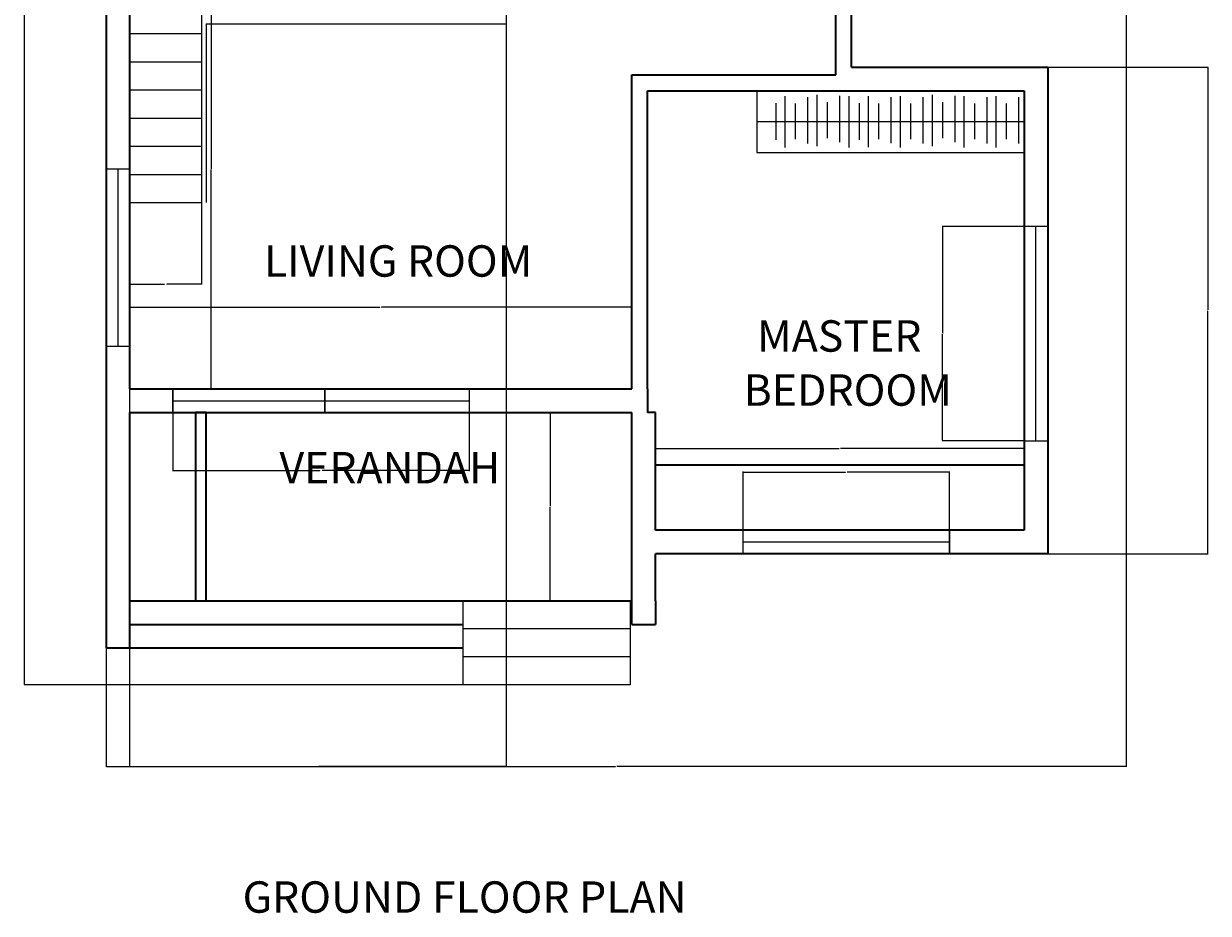
# Model space of a CAD drawing. Units: inches. Extents: x 1741 to 3812, y 9290 to 10023.
# Tile 1 of 5: x 1741 to 2194, y 9290 to 9630. Entities that reach past the tile are written whole.
import ezdxf

# ---------------------------------------------------------------- set-up
doc = ezdxf.new("R2010")
doc.units = ezdxf.units.IN
doc.header["$MEASUREMENT"] = 0
for name, color, linetype, lineweight in [('A-ANNO-DIMS', 2, 'Continuous', 18), ('A-ANNO-TEXT', 7, 'Continuous', 25), ('A-AREA-IDEN', 7, 'Continuous', 18), ('A-FLOR-CASE', 9, 'Continuous', 18), ('A-FLOR-STRS', 3, 'Continuous', 18), ('A-GLAZ', 4, 'Continuous', 18), ('A-WALL', 7, 'Continuous', 35)]:
    doc.layers.add(name, color=color, linetype=linetype, lineweight=lineweight)
doc.styles.get("Standard").update_dxf_attribs({"font": 'arial.ttf'})
doc.dimstyles.get("Standard").update_dxf_attribs({"dimtxt": 0.18, "dimasz": 0.18, "dimexe": 0.18, "dimexo": 0.0625, "dimgap": 0.09, "dimtad": 0, "dimtih": 1, "dimtoh": 1, "dimdec": 4, "dimzin": 0, "dimdsep": 46, "dimtxsty": 'Standard', "dimcen": 0.09, "dimadec": 0, "dimazin": 0, "dimtfac": 1, "dimtdec": 4, "dimtofl": 0, "dimtmove": 0, "dimatfit": 3, "dimfxl": 1, "dimtolj": 1, "dimtzin": 0, "dimarcsym": 0})

# ---------------------------------------------------------------- blocks, each defined once
blk = doc.blocks.new('*D31')
at = {"layer": 'A-ANNO-DIMS', "color": 0, "lineweight": -2, "transparency": 16777216}
for p, q in [((2162.92, 9640.39), (2162.92, 9345.97)), ((1772.92, 9391.39), (1772.92, 9345.97)), ((1773.1, 9346.15), (1967.64, 9346.15)), ((2162.74, 9346.15), (1968.21, 9346.15))]:
    blk.add_line(p, q, dxfattribs=at)
at = {"layer": 'A-ANNO-DIMS', "color": 0, "transparency": 16777216}
for points in [[(1773.1, 9346.18), (1773.1, 9346.12), (1772.92, 9346.15)], [(2162.74, 9346.18), (2162.74, 9346.12), (2162.92, 9346.15)]]:
    blk.add_solid(points, dxfattribs=at)
at = {"layer": 'Defpoints', "color": 0, "transparency": 16777216}
for p in [(2162.92, 9640.45), (1772.92, 9391.45), (2162.92, 9346.15)]:
    blk.add_point(p, dxfattribs=at)
at = {"layer": 'A-ANNO-DIMS', "color": 0, "transparency": 16777216, "insert": (1967.92, 9346.15), "char_height": 0.18, "attachment_point": 5}
blk.add_mtext('\\A1;390', dxfattribs=at)
blk = doc.blocks.new('*D32')
at = {"layer": 'A-ANNO-DIMS', "color": 0, "lineweight": -2, "transparency": 16777216}
for p, q in [((1844.86, 9901.45), (1741.54, 9901.45)), ((1741.72, 9901.27), (1741.72, 9639.58)), ((1741.72, 9377.53), (1741.72, 9639.22)), ((1909.43, 9377.35), (1741.54, 9377.35))]:
    blk.add_line(p, q, dxfattribs=at)
at = {"layer": 'A-ANNO-DIMS', "color": 0, "transparency": 16777216}
for points in [[(1741.69, 9901.27), (1741.75, 9901.27), (1741.72, 9901.45)], [(1741.69, 9377.53), (1741.75, 9377.53), (1741.72, 9377.35)]]:
    blk.add_solid(points, dxfattribs=at)
at = {"layer": 'Defpoints', "color": 0, "transparency": 16777216}
for p in [(1741.72, 9901.45), (1844.92, 9901.45), (1909.49, 9377.35)]:
    blk.add_point(p, dxfattribs=at)
at = {"layer": 'A-ANNO-DIMS', "color": 0, "transparency": 16777216, "insert": (1741.72, 9639.4), "char_height": 0.18, "attachment_point": 5}
blk.add_mtext('\\A1;524.1', dxfattribs=at)
blk = doc.blocks.new('*D41')
at = {"layer": 'A-ANNO-DIMS', "color": 0, "lineweight": -2, "transparency": 16777216}
for p, q in [((2132.99, 9613.45), (2194.3, 9613.45)), ((2194.12, 9613.27), (2194.12, 9520.63)), ((2194.12, 9427.63), (2194.12, 9520.27)), ((2132.99, 9427.45), (2194.3, 9427.45))]:
    blk.add_line(p, q, dxfattribs=at)
at = {"layer": 'A-ANNO-DIMS', "color": 0, "transparency": 16777216}
for points in [[(2194.09, 9613.27), (2194.15, 9613.27), (2194.12, 9613.45)], [(2194.09, 9427.63), (2194.15, 9427.63), (2194.12, 9427.45)]]:
    blk.add_solid(points, dxfattribs=at)
at = {"layer": 'Defpoints', "color": 0, "transparency": 16777216}
for p in [(2132.92, 9613.45), (2132.92, 9427.45), (2194.12, 9427.45)]:
    blk.add_point(p, dxfattribs=at)
at = {"layer": 'A-ANNO-DIMS', "color": 0, "transparency": 16777216, "insert": (2194.12, 9520.45), "char_height": 0.18, "attachment_point": 5}
blk.add_mtext('\\A1;186', dxfattribs=at)
blk = doc.blocks.new('*D42')
at = {"layer": 'A-ANNO-DIMS', "color": 0, "lineweight": -2, "transparency": 16777216}
for p, q in [((1781.92, 9832.39), (1781.92, 9345.97)), ((1925.92, 9832.39), (1925.92, 9345.97)), ((1782.1, 9346.15), (1853.64, 9346.15)), ((1925.74, 9346.15), (1854.2, 9346.15))]:
    blk.add_line(p, q, dxfattribs=at)
at = {"layer": 'A-ANNO-DIMS', "color": 0, "transparency": 16777216}
for points in [[(1782.1, 9346.18), (1782.1, 9346.12), (1781.92, 9346.15)], [(1925.74, 9346.18), (1925.74, 9346.12), (1925.92, 9346.15)]]:
    blk.add_solid(points, dxfattribs=at)
at = {"layer": 'Defpoints', "color": 0, "transparency": 16777216}
for p in [(1781.92, 9832.45), (1925.92, 9832.45), (1925.92, 9346.15)]:
    blk.add_point(p, dxfattribs=at)
at = {"layer": 'A-ANNO-DIMS', "color": 0, "transparency": 16777216, "insert": (1853.92, 9346.15), "char_height": 0.18, "attachment_point": 5}
blk.add_mtext('\\A1;144', dxfattribs=at)
blk = doc.blocks.new('*D47')
at = {"layer": 'A-ANNO-DIMS', "color": 0, "lineweight": -2, "transparency": 16777216}
for p, q in [((1781.92, 9490.51), (1781.92, 9521.83)), ((1782.1, 9521.65), (1877.64, 9521.65)), ((1973.74, 9521.65), (1878.2, 9521.65)), ((1973.92, 9490.51), (1973.92, 9521.83))]:
    blk.add_line(p, q, dxfattribs=at)
at = {"layer": 'A-ANNO-DIMS', "color": 0, "transparency": 16777216}
for points in [[(1782.1, 9521.68), (1782.1, 9521.62), (1781.92, 9521.65)], [(1973.74, 9521.68), (1973.74, 9521.62), (1973.92, 9521.65)]]:
    blk.add_solid(points, dxfattribs=at)
at = {"layer": 'Defpoints', "color": 0, "transparency": 16777216}
for p in [(1973.92, 9521.65), (1781.92, 9490.45), (1973.92, 9490.45)]:
    blk.add_point(p, dxfattribs=at)
at = {"layer": 'A-ANNO-DIMS', "color": 0, "transparency": 16777216, "insert": (1877.92, 9521.65), "char_height": 0.18, "attachment_point": 5}
blk.add_mtext('\\A1;192', dxfattribs=at)
blk = doc.blocks.new('*D48')
at = {"layer": 'A-ANNO-DIMS', "color": 0, "lineweight": -2, "transparency": 16777216}
for p, q in [((1781.99, 9658.45), (1813.3, 9658.45)), ((1813.12, 9658.27), (1813.12, 9574.63)), ((1813.12, 9490.63), (1813.12, 9574.27)), ((1781.99, 9490.45), (1813.3, 9490.45))]:
    blk.add_line(p, q, dxfattribs=at)
at = {"layer": 'A-ANNO-DIMS', "color": 0, "transparency": 16777216}
for points in [[(1813.09, 9658.27), (1813.15, 9658.27), (1813.12, 9658.45)], [(1813.09, 9490.63), (1813.15, 9490.63), (1813.12, 9490.45)]]:
    blk.add_solid(points, dxfattribs=at)
at = {"layer": 'Defpoints', "color": 0, "transparency": 16777216}
for p in [(1781.92, 9658.45), (1781.92, 9490.45), (1813.12, 9490.45)]:
    blk.add_point(p, dxfattribs=at)
at = {"layer": 'A-ANNO-DIMS', "color": 0, "transparency": 16777216, "insert": (1813.12, 9574.45), "char_height": 0.18, "attachment_point": 5}
blk.add_mtext('\\A1;168', dxfattribs=at)
blk = doc.blocks.new('*D49')
at = {"layer": 'A-ANNO-DIMS', "color": 0, "lineweight": -2, "transparency": 16777216}
for p, q in [((1982.92, 9436.51), (1982.92, 9467.83)), ((1983.1, 9467.65), (2053.16, 9467.65)), ((2123.74, 9467.65), (2053.69, 9467.65)), ((2123.92, 9436.51), (2123.92, 9467.83))]:
    blk.add_line(p, q, dxfattribs=at)
at = {"layer": 'A-ANNO-DIMS', "color": 0, "transparency": 16777216}
for points in [[(1983.1, 9467.68), (1983.1, 9467.62), (1982.92, 9467.65)], [(2123.74, 9467.68), (2123.74, 9467.62), (2123.92, 9467.65)]]:
    blk.add_solid(points, dxfattribs=at)
at = {"layer": 'Defpoints', "color": 0, "transparency": 16777216}
for p in [(2123.92, 9467.65), (1982.92, 9436.45), (2123.92, 9436.45)]:
    blk.add_point(p, dxfattribs=at)
at = {"layer": 'A-ANNO-DIMS', "color": 0, "transparency": 16777216, "insert": (2053.42, 9467.65), "char_height": 0.18, "attachment_point": 5}
blk.add_mtext('\\A1;141', dxfattribs=at)
blk = doc.blocks.new('*D50')
at = {"layer": 'A-ANNO-DIMS', "color": 0, "lineweight": -2, "transparency": 16777216}
for p, q in [((1973.86, 9481.45), (1942.54, 9481.45)), ((1942.72, 9481.27), (1942.72, 9445.63)), ((1942.72, 9409.63), (1942.72, 9445.27)), ((1973.86, 9409.45), (1942.54, 9409.45))]:
    blk.add_line(p, q, dxfattribs=at)
at = {"layer": 'A-ANNO-DIMS', "color": 0, "transparency": 16777216}
for points in [[(1942.69, 9481.27), (1942.75, 9481.27), (1942.72, 9481.45)], [(1942.69, 9409.63), (1942.75, 9409.63), (1942.72, 9409.45)]]:
    blk.add_solid(points, dxfattribs=at)
at = {"layer": 'Defpoints', "color": 0, "transparency": 16777216}
for p in [(1942.72, 9481.45), (1973.92, 9481.45), (1973.92, 9409.45)]:
    blk.add_point(p, dxfattribs=at)
at = {"layer": 'A-ANNO-DIMS', "color": 0, "transparency": 16777216, "insert": (1942.72, 9445.45), "char_height": 0.18, "attachment_point": 5}
blk.add_mtext('\\A1;72', dxfattribs=at)
blk = doc.blocks.new('*D51')
at = {"layer": 'A-ANNO-DIMS', "color": 0, "lineweight": -2, "transparency": 16777216}
for p, q in [((1781.92, 9561.63), (1781.92, 9530.32)), ((1809.45, 9561.63), (1809.45, 9530.32)), ((1782.1, 9530.5), (1795.22, 9530.5)), ((1809.27, 9530.5), (1796.15, 9530.5))]:
    blk.add_line(p, q, dxfattribs=at)
at = {"layer": 'A-ANNO-DIMS', "color": 0, "transparency": 16777216}
for points in [[(1782.1, 9530.53), (1782.1, 9530.47), (1781.92, 9530.5)], [(1809.27, 9530.53), (1809.27, 9530.47), (1809.45, 9530.5)]]:
    blk.add_solid(points, dxfattribs=at)
at = {"layer": 'Defpoints', "color": 0, "transparency": 16777216}
for p in [(1781.92, 9561.7), (1809.45, 9561.7), (1781.92, 9530.5)]:
    blk.add_point(p, dxfattribs=at)
at = {"layer": 'A-ANNO-DIMS', "color": 0, "transparency": 16777216, "insert": (1795.69, 9530.5), "char_height": 0.18, "attachment_point": 5}
blk.add_mtext('\\A1;27.524', dxfattribs=at)
blk = doc.blocks.new('*D53')
at = {"layer": 'A-ANNO-DIMS', "color": 0, "lineweight": -2, "transparency": 16777216}
for p, q in [((2016.46, 9427.51), (2016.46, 9458.83)), ((2016.64, 9458.65), (2055.59, 9458.65)), ((2095.18, 9458.65), (2056.23, 9458.65)), ((2095.36, 9427.51), (2095.36, 9458.83))]:
    blk.add_line(p, q, dxfattribs=at)
at = {"layer": 'A-ANNO-DIMS', "color": 0, "transparency": 16777216}
for points in [[(2016.64, 9458.68), (2016.64, 9458.62), (2016.46, 9458.65)], [(2095.18, 9458.68), (2095.18, 9458.62), (2095.36, 9458.65)]]:
    blk.add_solid(points, dxfattribs=at)
at = {"layer": 'Defpoints', "color": 0, "transparency": 16777216}
for p in [(2095.36, 9458.65), (2016.46, 9427.45), (2095.36, 9427.45)]:
    blk.add_point(p, dxfattribs=at)
at = {"layer": 'A-ANNO-DIMS', "color": 0, "transparency": 16777216, "insert": (2055.91, 9458.65), "char_height": 0.18, "attachment_point": 5}
blk.add_mtext('\\A1;78.9', dxfattribs=at)
blk = doc.blocks.new('*D54')
at = {"layer": 'A-ANNO-DIMS', "color": 0, "lineweight": -2, "transparency": 16777216}
for p, q in [((2123.86, 9552.56), (2092.54, 9552.56)), ((2092.72, 9552.38), (2092.72, 9511.78)), ((2092.72, 9470.81), (2092.72, 9511.41)), ((2123.86, 9470.63), (2092.54, 9470.63))]:
    blk.add_line(p, q, dxfattribs=at)
at = {"layer": 'A-ANNO-DIMS', "color": 0, "transparency": 16777216}
for points in [[(2092.69, 9552.38), (2092.75, 9552.38), (2092.72, 9552.56)], [(2092.69, 9470.81), (2092.75, 9470.81), (2092.72, 9470.63)]]:
    blk.add_solid(points, dxfattribs=at)
at = {"layer": 'Defpoints', "color": 0, "transparency": 16777216}
for p in [(2092.72, 9552.56), (2123.92, 9552.56), (2123.92, 9470.63)]:
    blk.add_point(p, dxfattribs=at)
at = {"layer": 'A-ANNO-DIMS', "color": 0, "transparency": 16777216, "insert": (2092.72, 9511.6), "char_height": 0.18, "attachment_point": 5}
blk.add_mtext('\\A1;81.93', dxfattribs=at)
blk = doc.blocks.new('*D55')
at = {"layer": 'A-ANNO-DIMS', "color": 0, "lineweight": -2, "transparency": 16777216}
for p, q in [((1798.4, 9490.39), (1798.4, 9459.07)), ((1911.72, 9490.39), (1911.72, 9459.07)), ((1798.58, 9459.25), (1854.6, 9459.25)), ((1911.54, 9459.25), (1855.51, 9459.25))]:
    blk.add_line(p, q, dxfattribs=at)
at = {"layer": 'A-ANNO-DIMS', "color": 0, "transparency": 16777216}
for points in [[(1798.58, 9459.28), (1798.58, 9459.22), (1798.4, 9459.25)], [(1911.54, 9459.28), (1911.54, 9459.22), (1911.72, 9459.25)]]:
    blk.add_solid(points, dxfattribs=at)
at = {"layer": 'Defpoints', "color": 0, "transparency": 16777216}
for p in [(1798.4, 9490.45), (1911.72, 9490.45), (1798.4, 9459.25)]:
    blk.add_point(p, dxfattribs=at)
at = {"layer": 'A-ANNO-DIMS', "color": 0, "transparency": 16777216, "insert": (1855.06, 9459.25), "char_height": 0.18, "attachment_point": 5}
blk.add_mtext('\\A1;113.32', dxfattribs=at)

msp = doc.modelspace()

# ---------------------------------------------------------------- linework, layer by layer
at = {"layer": 'A-FLOR-CASE'}
for p, q in [((2032.4394, 9602.3162), (2032.4394, 9582.7787)), ((2041.1456, 9601.9476), (2041.1456, 9584.3269)), ((2044.6351, 9602.8048), (2044.6351, 9583.2673)), ((2053.3413, 9602.4362), (2053.3413, 9584.8156)), ((2056.8308, 9602.3162), (2056.8308, 9582.7787)), ((2064.3045, 9602.3625), (2064.3045, 9582.825)), ((2073.0107, 9601.9939), (2073.0107, 9584.3732)), ((2076.5002, 9602.3162), (2076.5002, 9582.7787)), ((2085.2063, 9601.9476), (2085.2063, 9584.3269)), ((2088.6959, 9602.8048), (2088.6959, 9583.2673)), ((2097.402, 9602.4362), (2097.402, 9584.8156)), ((2100.8916, 9602.3162), (2100.8916, 9582.7787)), ((2109.5977, 9601.9476), (2109.5977, 9584.3269)), ((2113.0872, 9602.3162), (2113.0872, 9582.7787)), ((2121.7934, 9601.9476), (2121.7934, 9584.3269)), ((2028.9499, 9599.6479), (2028.9499, 9585.6492)), ((2036.4236, 9599.5146), (2036.4236, 9585.8752)), ((2041.1456, 9600.1366), (2041.1456, 9586.1379)), ((2048.6193, 9600.0033), (2048.6193, 9586.3638)), ((2053.3413, 9599.6479), (2053.3413, 9585.6492)), ((2060.815, 9599.6942), (2060.815, 9585.6955)), ((2060.815, 9599.5146), (2060.815, 9585.8752)), ((2068.2887, 9599.5609), (2068.2887, 9585.9215)), ((2073.0107, 9599.6479), (2073.0107, 9585.6492)), ((2080.4843, 9599.5146), (2080.4843, 9585.8752)), ((2085.2063, 9600.1366), (2085.2063, 9586.1379)), ((2092.68, 9600.0033), (2092.68, 9586.3638)), ((2097.402, 9599.6479), (2097.402, 9585.6492)), ((2104.8757, 9599.5146), (2104.8757, 9585.8752)), ((2109.5977, 9599.6479), (2109.5977, 9585.6492)), ((2117.0714, 9599.5146), (2117.0714, 9585.8752)), ((2021.6546, 9592.6486), (2123.9242, 9592.6486))]:
    msp.add_line(p, q, dxfattribs=at)
msp.add_lwpolyline([(2123.9242, 9604.4507), (2021.6546, 9604.4507), (2021.6546, 9580.8465), (2123.9242, 9580.8465)], close=True, dxfattribs=at)
at = {"layer": 'A-FLOR-STRS'}
for p, q in [((1925.9242, 9658.4507), (1925.9242, 9630.0587)), ((1809.4485, 9637.0717), (1809.4485, 9561.6958)), ((1811.2454, 9630.0587), (1811.2454, 9561.6958)), ((1811.2454, 9630.0587), (1925.9242, 9630.0587)), ((1781.9242, 9626.3037), (1809.4485, 9626.3037)), ((1781.9242, 9615.5357), (1809.4485, 9615.5357)), ((1781.9242, 9604.7678), (1809.4485, 9604.7678)), ((1781.9242, 9593.9998), (1809.4485, 9593.9998)), ((1781.9242, 9583.2318), (1809.4485, 9583.2318)), ((1781.9242, 9572.4638), (1809.4485, 9572.4638)), ((1781.9242, 9561.6958), (1809.4485, 9561.6958)), ((1909.4893, 9409.4507), (1973.3224, 9409.4507)), ((1909.4893, 9377.3522), (1909.4893, 9409.4507)), ((1973.3224, 9409.4507), (1909.4893, 9409.4507)), ((1973.3224, 9409.4507), (1973.3224, 9377.3522)), ((1973.3224, 9398.7512), (1909.4893, 9398.7512)), ((1973.3224, 9388.0517), (1909.4893, 9388.0517)), ((1973.3224, 9377.3522), (1909.4893, 9377.3522))]:
    msp.add_line(p, q, dxfattribs=at)
at = {"layer": 'A-GLAZ'}
for p, q in [((1777.4242, 9574.4507), (1777.4242, 9506.7599)), ((2128.4242, 9470.6302), (2128.4242, 9552.5627)), ((1798.4, 9485.9507), (1911.7153, 9485.9507)), ((2016.4607, 9431.9507), (2095.3581, 9431.9507))]:
    msp.add_line(p, q, dxfattribs=at)
for points in [[(1781.9242, 9574.4507), (1772.9242, 9574.4507), (1772.9242, 9506.7599), (1781.9242, 9506.7599)], [(2132.9242, 9552.5627), (2123.9242, 9552.5627), (2123.9242, 9470.6302), (2132.9242, 9470.6302)], [(1798.4, 9490.4507), (1856.4884, 9490.4507), (1856.4884, 9481.4507), (1798.4, 9481.4507)], [(1856.4884, 9490.4507), (1911.7153, 9490.4507), (1911.7153, 9481.4507), (1856.4884, 9481.4507)], [(2016.4607, 9436.4507), (2095.3581, 9436.4507), (2095.3581, 9427.4507), (2016.4607, 9427.4507)]]:
    msp.add_lwpolyline(points, close=True, dxfattribs=at)
at = {"layer": 'A-WALL'}
for p, q in [((2051.9242, 9610.4507), (2051.9242, 9712.4507)), ((1772.9242, 9658.4507), (1772.9242, 9490.4507)), ((1781.9242, 9658.4507), (1781.9242, 9490.4507)), ((2057.9242, 9613.4507), (2057.9242, 9640.4507)), ((2057.9242, 9613.4507), (2132.9242, 9613.4507)), ((2132.9242, 9613.4507), (2132.9242, 9427.4507)), ((1973.9242, 9610.4507), (2051.9242, 9610.4507)), ((1973.9242, 9490.4507), (1973.9242, 9610.4507)), ((1979.9242, 9490.4507), (1979.9242, 9604.4507)), ((1979.9242, 9604.4507), (2123.9242, 9604.4507)), ((1979.9242, 9604.4507), (2051.9242, 9604.4507)), ((2123.9242, 9604.4507), (2123.9242, 9436.4507)), ((1772.9242, 9490.4507), (1772.9242, 9481.4507)), ((1781.9242, 9490.4507), (1973.9242, 9490.4507)), ((1979.9242, 9490.4507), (1979.9242, 9481.4507)), ((1772.9242, 9481.4507), (1772.9242, 9391.4507)), ((1781.9242, 9481.4507), (1973.9242, 9481.4507)), ((1781.9242, 9481.4507), (1781.9242, 9391.4507)), ((1973.9242, 9400.4507), (1973.9242, 9481.4507)), ((1982.9242, 9481.4507), (1979.9242, 9481.4507)), ((1982.9242, 9436.4507), (1982.9242, 9481.4507)), ((2123.9242, 9461.3434), (1982.9242, 9461.3434)), ((2123.9242, 9436.4507), (1982.9242, 9436.4507)), ((1982.9242, 9409.4507), (1982.9242, 9427.4507)), ((2132.9242, 9427.4507), (1982.9242, 9427.4507)), ((1781.9242, 9409.4507), (1973.9242, 9409.4507)), ((1982.9242, 9409.4507), (1982.9242, 9400.4507)), ((1781.9242, 9400.4507), (1909.4893, 9400.4507)), ((1973.9242, 9400.4507), (1982.9242, 9400.4507)), ((1772.9242, 9391.4507), (1909.4893, 9391.4507))]:
    msp.add_line(p, q, dxfattribs=at)
msp.add_lwpolyline([(1811.1189, 9481.4507), (1807.0567, 9481.4507), (1807.0567, 9409.4507), (1811.1189, 9409.4507)], close=True, dxfattribs=at)

# ---------------------------------------------------------------- texts
at = {"layer": 'A-ANNO-TEXT'}
msp.add_text('GROUND FLOOR PLAN', height=12, dxfattribs=at).set_placement((1825.1118, 9290.2226))
at = {"layer": 'A-AREA-IDEN'}
for s, p in [('LIVING ROOM', (1833.2597, 9533.3552)), (' MASTER ', (2018.1154, 9504.6919)), ('BEDROOM', (2016.6786, 9484.0171)), ('VERANDAH', (1839.211, 9454.3263))]:
    msp.add_text(s, height=12, dxfattribs=at).set_placement(p)

# ---------------------------------------------------------------- dimensions: what is measured, and where the dimension line sits
at = {"layer": 'A-ANNO-DIMS'}
for base, p1, p2, angle, override, picture, middle in [((1741.7242, 9901.4507), (1909.4893, 9377.3522), (1844.9242, 9901.4507), 90, {"dimdec": 1, "dimlfac": 1, "dimrnd": 0, "dimzin": 0, "dimdsep": 46, "dimlunit": 2}, '*D32', (1741.7242, 9639.4015)), ((1813.1242, 9490.4507), (1781.9242, 9658.4507), (1781.9242, 9490.4507), 270, {"dimdec": 0, "dimlfac": 1, "dimrnd": 0, "dimzin": 0, "dimdsep": 46, "dimlunit": 2}, '*D48', (1813.1242, 9574.4507)), ((2194.1242, 9427.4507), (2132.9242, 9613.4507), (2132.9242, 9427.4507), 90, {"dimdec": 0, "dimlfac": 1, "dimrnd": 0, "dimzin": 0, "dimdsep": 46, "dimlunit": 2}, '*D41', (2194.1242, 9520.4507)), ((1781.9242, 9530.4958), (1809.4485, 9561.6958), (1781.9242, 9561.6958), 180, {"dimdec": 3, "dimlfac": 1, "dimrnd": 0, "dimzin": 0, "dimdsep": 46, "dimlunit": 2}, '*D51', (1795.6863, 9530.4958)), ((2092.7242, 9552.5627), (2123.9242, 9470.6302), (2123.9242, 9552.5627), 90, {"dimdec": 2, "dimlfac": 1, "dimrnd": 0, "dimzin": 0, "dimdsep": 46, "dimlunit": 2}, '*D54', (2092.7242, 9511.5965)), ((1798.4, 9459.2507), (1911.7153, 9490.4507), (1798.4, 9490.4507), 180, {"dimdec": 2, "dimlfac": 1, "dimrnd": 0, "dimzin": 0, "dimdsep": 46, "dimlunit": 2}, '*D55', (1855.0577, 9459.2507)), ((1942.7242, 9481.4507), (1973.9242, 9409.4507), (1973.9242, 9481.4507), 90, {"dimdec": 0, "dimlfac": 1, "dimrnd": 0, "dimzin": 0, "dimdsep": 46, "dimlunit": 2}, '*D50', (1942.7242, 9445.4507)), ((2123.9242, 9467.6507), (1982.9242, 9436.4507), (2123.9242, 9436.4507), 0, {"dimdec": 0, "dimlfac": 1, "dimrnd": 0, "dimzin": 0, "dimdsep": 46, "dimlunit": 2}, '*D49', (2053.4242, 9467.6507))]:
    dim = msp.add_linear_dim(base=base, p1=p1, p2=p2, angle=angle, dimstyle='Standard', override=override, dxfattribs=at)
    dim.commit()
    dim.dimension.update_dxf_attribs({"geometry": picture, "text_midpoint": middle})
for base, p1, p2, override, picture, middle in [((1925.9242, 9346.1522), (1781.9242, 9832.4507), (1925.9242, 9832.4507), {"dimdec": 0, "dimlfac": 1, "dimrnd": 0, "dimzin": 0, "dimdsep": 46, "dimlunit": 2}, '*D42', (1853.9242, 9346.1522)), ((2162.9242, 9346.1522), (1772.9242, 9391.4507), (2162.9242, 9640.4507), {"dimdec": 0, "dimlfac": 1, "dimrnd": 0, "dimzin": 0, "dimdsep": 46, "dimlunit": 2}, '*D31', (1967.9242, 9346.1522)), ((1973.9242, 9521.6507), (1781.9242, 9490.4507), (1973.9242, 9490.4507), {"dimdec": 0, "dimlfac": 1, "dimrnd": 0, "dimzin": 0, "dimdsep": 46, "dimlunit": 2}, '*D47', (1877.9242, 9521.6507)), ((2095.3581, 9458.6507), (2016.4607, 9427.4507), (2095.3581, 9427.4507), {"dimdec": 1, "dimlfac": 1, "dimrnd": 0, "dimzin": 0, "dimdsep": 46, "dimlunit": 2}, '*D53', (2055.9094, 9458.6507))]:
    dim = msp.add_linear_dim(base=base, p1=p1, p2=p2, dimstyle='Standard', override=override, dxfattribs=at)
    dim.commit()
    dim.dimension.update_dxf_attribs({"geometry": picture, "text_midpoint": middle})

doc.saveas('drawing.dxf')
